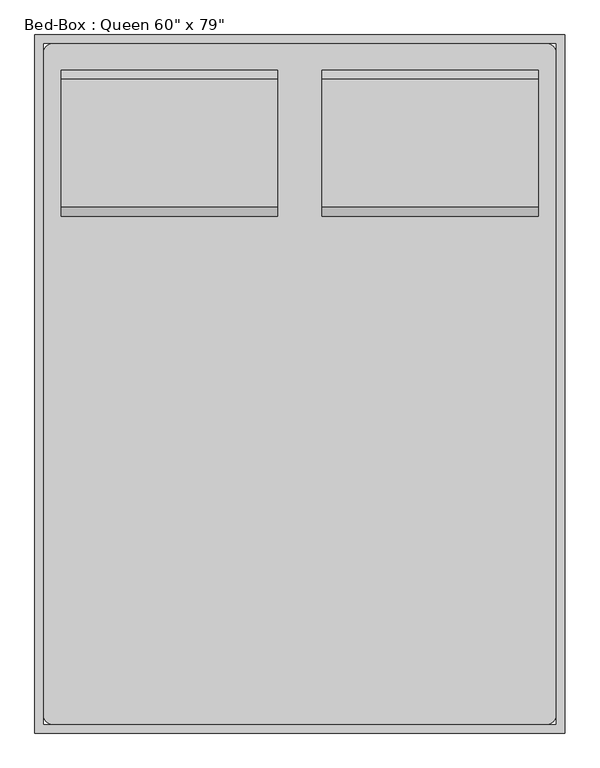
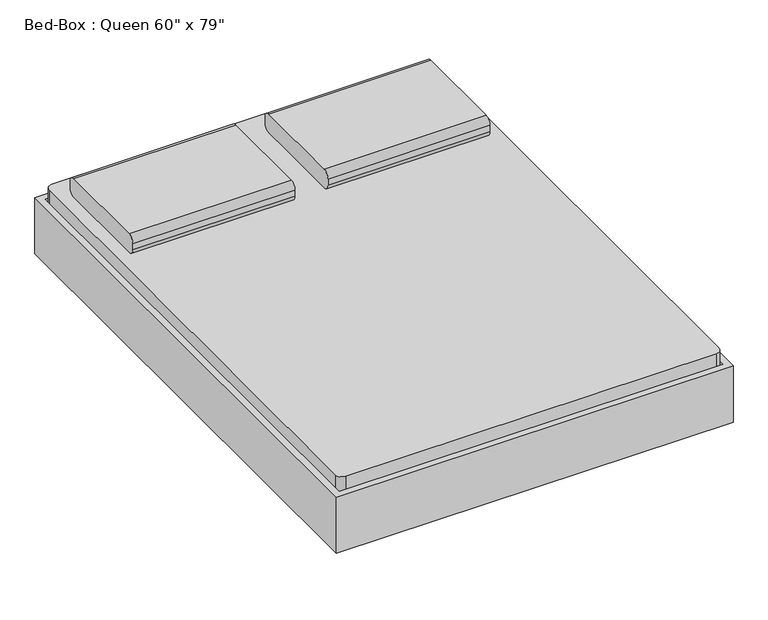
"""IFC4 building model written with IfcOpenShell, lengths in millimetres: furniture geometry."""

from ifc_helpers import new_model, si_unit, point, frame, frame_2d, origin, place, context, project, spatial, polyline, circle_curve, trimmed, segment, composite_curve, outline, extrude, source, transform, mapped, element, save
from ifc_brep_helpers import plane_surface, cylinder_surface, revolved_surface, advanced_brep


def furniture_1d2926bd(model_context):
    return source(origin(), model_context, "Body", "SolidModel", [
        extrude(outline(composite_curve([segment(polyline([(641.8704918, 406.4), (273.5704918, 406.4)]), True, "CONTINUOUS"), segment(trimmed(circle_curve(frame_2d((273.5704918, 431.8)), 25.4), [point((273.5704918, 406.4))], [point((248.1704918, 431.8))], False, "CARTESIAN"), True, "CONTINUOUS"), segment(polyline([(248.1704918, 431.8), (248.1704918, 457.2)]), True, "CONTINUOUS"), segment(trimmed(circle_curve(frame_2d((273.5704918, 457.2)), 25.4), [point((248.1704918, 457.2))], [point((273.5704918, 482.6))], False, "CARTESIAN"), True, "CONTINUOUS"), segment(polyline([(273.5704918, 482.6), (641.8704918, 482.6)]), True, "CONTINUOUS"), segment(trimmed(circle_curve(frame_2d((641.8704918, 457.2)), 25.4), [point((641.8704918, 482.6))], [point((667.2704918, 457.2))], False, "CARTESIAN"), True, "CONTINUOUS"), segment(polyline([(667.2704918, 457.2), (667.2704918, 431.8)]), True, "CONTINUOUS"), segment(trimmed(circle_curve(frame_2d((641.8704918, 431.8)), 25.4), [point((667.2704918, 431.8))], [point((641.8704918, 406.4))], False, "CARTESIAN"), True, "CONTINUOUS")], self_intersect=False)), frame((402.652459, 0.0, 0.0), z_axis=(1.0, 0.0, 0.0), x_axis=(0.0, 1.0, 0.0)), (0.0, 0.0, 1.0), 622.3),
        extrude(outline(composite_curve([segment(polyline([(641.8704918, 406.4), (273.5704918, 406.4)]), True, "CONTINUOUS"), segment(trimmed(circle_curve(frame_2d((273.5704918, 431.8)), 25.4), [point((273.5704918, 406.4))], [point((248.1704918, 431.8))], False, "CARTESIAN"), True, "CONTINUOUS"), segment(polyline([(248.1704918, 431.8), (248.1704918, 457.2)]), True, "CONTINUOUS"), segment(trimmed(circle_curve(frame_2d((273.5704918, 457.2)), 25.4), [point((248.1704918, 457.2))], [point((273.5704918, 482.6))], False, "CARTESIAN"), True, "CONTINUOUS"), segment(polyline([(273.5704918, 482.6), (641.8704918, 482.6)]), True, "CONTINUOUS"), segment(trimmed(circle_curve(frame_2d((641.8704918, 457.2)), 25.4), [point((641.8704918, 482.6))], [point((667.2704918, 457.2))], False, "CARTESIAN"), True, "CONTINUOUS"), segment(polyline([(667.2704918, 457.2), (667.2704918, 431.8)]), True, "CONTINUOUS"), segment(trimmed(circle_curve(frame_2d((641.8704918, 431.8)), 25.4), [point((667.2704918, 431.8))], [point((641.8704918, 406.4))], False, "CARTESIAN"), True, "CONTINUOUS")], self_intersect=False)), frame((-346.647541, 0.0, 0.0), z_axis=(1.0, 0.0, 0.0), x_axis=(0.0, 1.0, 0.0)), (0.0, 0.0, 1.0), 622.3),
        advanced_brep(
        [(-397.1231784, 514.8704918, 177.8), (-397.1231784, 438.6704918, 177.8), (-397.1231784, 438.6704918, 196.85), (-397.1231784, 514.8704918, 196.85), (-346.3231784, 514.8704918, 177.8), (-346.3231784, 438.6704918, 177.8), (-334.1869899, 438.6704918, 196.85), (-334.1869899, 514.8704918, 196.85), (-270.2523099, 514.8704918, 14.6654962), (-270.2523099, 438.6704918, 14.6654962), (-252.9871466, 438.6704918, 22.716374), (-252.9871466, 514.8704918, 22.716374), (-247.2320921, 438.6704918, 0.0), (-247.2320921, 514.8704918, 0.0), (-247.2320921, 438.6704918, 19.05), (-247.2320921, 514.8704918, 19.05), (-168.6195862, 514.8704918, 0.0), (-168.6195862, 438.6704918, 0.0), (-168.6195862, 438.6704918, 19.05), (-168.6195862, 514.8704918, 19.05), (-155.9195862, 438.6704918, 3.4029547), (-155.9195862, 514.8704918, 3.4029547), (-165.4445862, 438.6704918, 19.9007387), (-165.4445862, 514.8704918, 19.9007387), (-95.822541, 514.8704918, 38.1), (-95.822541, 438.6704918, 38.1), (-100.9269731, 438.6704918, 57.15), (-100.9269731, 514.8704918, 57.15), (774.4518216, 514.8704918, 38.1), (774.4518216, 438.6704918, 38.1), (779.5562537, 438.6704918, 57.15), (779.5562537, 514.8704918, 57.15), (834.5488669, 514.8704918, 3.4029547), (834.5488669, 438.6704918, 3.4029547), (844.0738669, 438.6704918, 19.9007387), (844.0738669, 514.8704918, 19.9007387), (847.2488669, 438.6704918, 0.0), (847.2488669, 514.8704918, 0.0), (847.2488669, 438.6704918, 19.05), (847.2488669, 514.8704918, 19.05), (925.8613728, 514.8704918, 0.0), (925.8613728, 438.6704918, 0.0), (925.8613728, 438.6704918, 19.05), (925.8613728, 514.8704918, 19.05), (948.8815906, 438.6704918, 14.6654962), (948.8815906, 514.8704918, 14.6654962), (931.6164272, 438.6704918, 22.716374), (931.6164272, 514.8704918, 22.716374), (1024.952459, 514.8704918, 177.8), (1024.952459, 438.6704918, 177.8), (1012.8162705, 438.6704918, 196.85), (1012.8162705, 514.8704918, 196.85), (1075.752459, 514.8704918, 177.8), (1075.752459, 514.8704918, 196.85), (1075.752459, 438.6704918, 196.85), (1075.752459, 438.6704918, 177.8)],
        [
            (0, 1),
            (1, 2),
            (2, 3),
            (3, 0),
            (0, 4),
            (4, 5),
            (5, 1),
            (5, 6),
            (6, 2),
            (6, 7),
            (7, 3),
            (7, 4),
            (4, 8),
            (8, 9),
            (9, 5),
            (9, 10),
            (10, 6),
            (10, 11),
            (11, 7),
            (11, 8),
            (12, 9, circle_curve(frame((-247.2320921, 438.6704918, 25.4), z_axis=(0.0, 1.0, 0.0), x_axis=(-0.9063077870366486, 0.0, -0.42261826174070233)), 25.4)),
            (8, 13, circle_curve(frame((-247.2320921, 514.8704918, 25.4), z_axis=(0.0, -1.0, 0.0), x_axis=(-0.9063077870366486, 0.0, -0.42261826174070233)), 25.4)),
            (13, 12),
            (14, 10, circle_curve(frame((-247.2320921, 438.6704918, 25.4), z_axis=(0.0, 1.0, 0.0), x_axis=(-0.9063077870366486, 0.0, -0.42261826174070233)), 6.35)),
            (12, 14),
            (15, 11, circle_curve(frame((-247.2320921, 514.8704918, 25.4), z_axis=(0.0, 1.0, 0.0), x_axis=(-0.9063077870366486, 0.0, -0.42261826174070233)), 6.35)),
            (14, 15),
            (15, 13),
            (13, 16),
            (16, 17),
            (17, 12),
            (17, 18),
            (18, 14),
            (18, 19),
            (19, 15),
            (19, 16),
            (20, 17, circle_curve(frame((-168.6195862, 438.6704918, 25.4), z_axis=(0.0, 1.0, 0.0), x_axis=(0.0, 0.0, -1.0)), 25.4)),
            (16, 21, circle_curve(frame((-168.6195862, 514.8704918, 25.4), z_axis=(0.0, -1.0, 0.0), x_axis=(0.0, 0.0, -1.0)), 25.4)),
            (21, 20),
            (22, 18, circle_curve(frame((-168.6195862, 438.6704918, 25.4), z_axis=(0.0, 1.0, 0.0), x_axis=(0.0, 0.0, -1.0)), 6.35)),
            (20, 22),
            (23, 19, circle_curve(frame((-168.6195862, 514.8704918, 25.4), z_axis=(0.0, 1.0, 0.0), x_axis=(0.0, 0.0, -1.0)), 6.35)),
            (22, 23),
            (23, 21),
            (21, 24),
            (24, 25),
            (25, 20),
            (25, 26),
            (26, 22),
            (26, 27),
            (27, 23),
            (27, 24),
            (24, 28),
            (28, 29),
            (29, 25),
            (29, 30),
            (30, 26),
            (30, 31),
            (31, 27),
            (31, 28),
            (28, 32),
            (32, 33),
            (33, 29),
            (33, 34),
            (34, 30),
            (34, 35),
            (35, 31),
            (35, 32),
            (36, 33, circle_curve(frame((847.2488669, 438.6704918, 25.4), z_axis=(0.0, 1.0, 0.0), x_axis=(-0.5000000000000463, 0.0, -0.8660254037844118)), 25.4)),
            (32, 37, circle_curve(frame((847.2488669, 514.8704918, 25.4), z_axis=(0.0, -1.0, 0.0), x_axis=(-0.5000000000000463, 0.0, -0.8660254037844118)), 25.4)),
            (37, 36),
            (38, 34, circle_curve(frame((847.2488669, 438.6704918, 25.4), z_axis=(0.0, 1.0, 0.0), x_axis=(-0.5000000000000463, 0.0, -0.8660254037844118)), 6.35)),
            (36, 38),
            (39, 35, circle_curve(frame((847.2488669, 514.8704918, 25.4), z_axis=(0.0, 1.0, 0.0), x_axis=(-0.5000000000000463, 0.0, -0.8660254037844118)), 6.35)),
            (38, 39),
            (39, 37),
            (37, 40),
            (40, 41),
            (41, 36),
            (41, 42),
            (42, 38),
            (42, 43),
            (43, 39),
            (43, 40),
            (44, 41, circle_curve(frame((925.8613728, 438.6704918, 25.4), z_axis=(0.0, 1.0, 0.0), x_axis=(0.0, 0.0, -1.0)), 25.4)),
            (40, 45, circle_curve(frame((925.8613728, 514.8704918, 25.4), z_axis=(0.0, -1.0, 0.0), x_axis=(0.0, 0.0, -1.0)), 25.4)),
            (45, 44),
            (46, 42, circle_curve(frame((925.8613728, 438.6704918, 25.4), z_axis=(0.0, 1.0, 0.0), x_axis=(0.0, 0.0, -1.0)), 6.35)),
            (44, 46),
            (47, 43, circle_curve(frame((925.8613728, 514.8704918, 25.4), z_axis=(0.0, 1.0, 0.0), x_axis=(0.0, 0.0, -1.0)), 6.35)),
            (46, 47),
            (47, 45),
            (45, 48),
            (48, 49),
            (49, 44),
            (49, 50),
            (50, 46),
            (50, 51),
            (51, 47),
            (51, 48),
            (52, 53),
            (53, 54),
            (54, 55),
            (55, 52),
            (48, 52),
            (55, 49),
            (54, 50),
            (53, 51),
        ],
        [
            plane_surface(frame((-397.1231784, 768.8704918, -152.9490627), z_axis=(-1.0, 0.0, 0.0), x_axis=(0.0, 1.0, 0.0))),
            plane_surface(frame((-397.1231784, 514.8704918, 177.8), z_axis=(0.0, 0.0, -1.0), x_axis=(1.0, 0.0, 0.0))),
            plane_surface(frame((-397.1231784, 438.6704918, 177.8), z_axis=(0.0, -1.0, 0.0), x_axis=(1.0, 0.0, 0.0))),
            plane_surface(frame((-397.1231784, 438.6704918, 196.85), z_axis=(0.0, 0.0, 1.0), x_axis=(1.0, 0.0, 0.0))),
            plane_surface(frame((-397.1231784, 514.8704918, 196.85), z_axis=(0.0, 1.0, 0.0), x_axis=(1.0, 0.0, 0.0))),
            plane_surface(frame((-346.3231784, 514.8704918, 177.8), z_axis=(-0.9063077870366485, 0.0, -0.4226182617407027), x_axis=(0.4226182617407027, 0.0, -0.9063077870366485))),
            plane_surface(frame((-346.3231784, 438.6704918, 177.8), z_axis=(0.0, -1.0, 0.0), x_axis=(0.4226182617407025, 0.0, -0.9063077870366486))),
            plane_surface(frame((-334.1869899, 438.6704918, 196.85), z_axis=(0.9063077870366484, 0.0, 0.4226182617407028), x_axis=(0.4226182617407028, 0.0, -0.9063077870366484))),
            plane_surface(frame((-334.1869899, 514.8704918, 196.85), z_axis=(0.0, 1.0, 0.0), x_axis=(0.42261826174070277, 0.0, -0.9063077870366485))),
            cylinder_surface(frame((-247.2320921, 768.8704918, 25.4), z_axis=(0.0, -1.0, 0.0), x_axis=(-0.9063077870366486, 0.0, -0.42261826174070233)), 25.4),
            plane_surface(frame((-247.2320921, 438.6704918, 25.4), z_axis=(0.0, -1.0, 0.0), x_axis=(-0.9063077870366486, 0.0, -0.42261826174070233))),
            revolved_surface(polyline([(-252.9871465476827, 438.6704918, 22.71637403794654), (-252.9871465476827, 514.8704918, 22.71637403794654)]), (-247.2320921, 768.8704918, 25.4), (0.0, -1.0, 0.0)),
            plane_surface(frame((-247.2320921, 514.8704918, 25.4), z_axis=(0.0, 1.0, 0.0), x_axis=(-0.9063077870366486, 0.0, -0.42261826174070233))),
            plane_surface(frame((-247.2320921, 514.8704918, 0.0), z_axis=(0.0, 0.0, -1.0), x_axis=(1.0, 0.0, 0.0))),
            plane_surface(frame((-247.2320921, 438.6704918, 0.0), z_axis=(0.0, -1.0, 0.0), x_axis=(1.0, 0.0, 0.0))),
            plane_surface(frame((-247.2320921, 438.6704918, 19.05), z_axis=(0.0, 0.0, 1.0), x_axis=(1.0, 0.0, 0.0))),
            plane_surface(frame((-247.2320921, 514.8704918, 19.05), z_axis=(0.0, 1.0, 0.0), x_axis=(1.0, 0.0, 0.0))),
            cylinder_surface(frame((-168.6195862, 768.8704918, 25.4), z_axis=(0.0, -1.0, 0.0), x_axis=(0.0, 0.0, -1.0)), 25.4),
            plane_surface(frame((-168.6195862, 438.6704918, 25.4), z_axis=(0.0, -1.0, 0.0), x_axis=(0.0, 0.0, -1.0))),
            revolved_surface(polyline([(-168.6195862, 438.6704918, 19.049999999999997), (-168.6195862, 514.8704918, 19.049999999999997)]), (-168.6195862, 768.8704918, 25.4), (0.0, -1.0, 0.0)),
            plane_surface(frame((-168.6195862, 514.8704918, 25.4), z_axis=(0.0, 1.0, 0.0), x_axis=(0.0, 0.0, -1.0))),
            plane_surface(frame((-155.9195862, 514.8704918, 3.4029547), z_axis=(0.49999999999988004, 0.0, -0.866025403784508), x_axis=(0.866025403784508, 0.0, 0.49999999999988004))),
            plane_surface(frame((-155.9195862, 438.6704918, 3.4029547), z_axis=(0.0, -1.0, 0.0), x_axis=(0.8660254037845078, 0.0, 0.49999999999988026))),
            plane_surface(frame((-165.4445862, 438.6704918, 19.9007387), z_axis=(-0.4999999999998799, 0.0, 0.866025403784508), x_axis=(0.866025403784508, 0.0, 0.4999999999998799))),
            plane_surface(frame((-165.4445862, 514.8704918, 19.9007387), z_axis=(0.0, 1.0, 0.0), x_axis=(0.8660254037845075, 0.0, 0.49999999999988076))),
            plane_surface(frame((-95.822541, 514.8704918, 38.1), z_axis=(0.0, 0.0, -1.0), x_axis=(1.0, 0.0, 0.0))),
            plane_surface(frame((-95.822541, 438.6704918, 38.1), z_axis=(0.0, -1.0, 0.0), x_axis=(1.0, 0.0, 0.0))),
            plane_surface(frame((-100.9269731, 438.6704918, 57.15), z_axis=(0.0, 0.0, 1.0), x_axis=(1.0, 0.0, 0.0))),
            plane_surface(frame((-100.9269731, 514.8704918, 57.15), z_axis=(0.0, 1.0, 0.0), x_axis=(1.0, 0.0, 0.0))),
            plane_surface(frame((774.4518216, 514.8704918, 38.1), z_axis=(-0.5000000000000455, 0.0, -0.8660254037844125), x_axis=(0.8660254037844125, 0.0, -0.5000000000000455))),
            plane_surface(frame((774.4518216, 438.6704918, 38.1), z_axis=(0.0, -1.0, 0.0), x_axis=(0.866025403784412, 0.0, -0.5000000000000463))),
            plane_surface(frame((779.5562537, 438.6704918, 57.15), z_axis=(0.5000000000000466, 0.0, 0.8660254037844117), x_axis=(0.8660254037844117, 0.0, -0.5000000000000466))),
            plane_surface(frame((779.5562537, 514.8704918, 57.15), z_axis=(0.0, 1.0, 0.0), x_axis=(0.8660254037844115, 0.0, -0.5000000000000471))),
            cylinder_surface(frame((847.2488669, 768.8704918, 25.4), z_axis=(0.0, -1.0, 0.0), x_axis=(-0.5000000000000463, 0.0, -0.8660254037844118)), 25.4),
            plane_surface(frame((847.2488669, 438.6704918, 25.4), z_axis=(0.0, -1.0000000000000002, 0.0), x_axis=(-0.5000000000000464, 0.0, -0.866025403784412))),
            revolved_surface(polyline([(844.0738668999998, 438.6704918, 19.90073868596898), (844.0738668999998, 514.8704918, 19.90073868596898)]), (847.2488669, 768.8704918, 25.4), (0.0, -1.0, 0.0)),
            plane_surface(frame((847.2488669, 514.8704918, 25.4), z_axis=(0.0, 1.0000000000000002, 0.0), x_axis=(-0.5000000000000464, 0.0, -0.866025403784412))),
            plane_surface(frame((847.2488669, 514.8704918, 0.0), z_axis=(0.0, 0.0, -1.0), x_axis=(1.0, 0.0, 0.0))),
            plane_surface(frame((847.2488669, 438.6704918, 0.0), z_axis=(0.0, -1.0, 0.0), x_axis=(1.0, 0.0, 0.0))),
            plane_surface(frame((847.2488669, 438.6704918, 19.05), z_axis=(0.0, 0.0, 1.0), x_axis=(1.0, 0.0, 0.0))),
            plane_surface(frame((847.2488669, 514.8704918, 19.05), z_axis=(0.0, 1.0, 0.0), x_axis=(1.0, 0.0, 0.0))),
            cylinder_surface(frame((925.8613728, 768.8704918, 25.4), z_axis=(0.0, -1.0, 0.0), x_axis=(0.0, 0.0, -1.0)), 25.4),
            plane_surface(frame((925.8613728, 438.6704918, 25.4), z_axis=(0.0, -1.0, 0.0), x_axis=(0.0, 0.0, -1.0))),
            revolved_surface(polyline([(925.8613728, 438.6704918, 19.049999999999997), (925.8613728, 514.8704918, 19.049999999999997)]), (925.8613728, 768.8704918, 25.4), (0.0, -1.0, 0.0)),
            plane_surface(frame((925.8613728, 514.8704918, 25.4), z_axis=(0.0, 1.0, 0.0), x_axis=(0.0, 0.0, -1.0))),
            plane_surface(frame((948.8815906, 514.8704918, 14.6654962), z_axis=(0.90630778703668, 0.0, -0.42261826174063505), x_axis=(0.42261826174063505, 0.0, 0.90630778703668))),
            plane_surface(frame((948.8815906, 438.6704918, 14.6654962), z_axis=(0.0, -1.0, 0.0), x_axis=(0.42261826174063566, 0.0, 0.9063077870366797))),
            plane_surface(frame((931.6164272, 438.6704918, 22.716374), z_axis=(-0.9063077870366801, 0.0, 0.42261826174063477), x_axis=(0.42261826174063477, 0.0, 0.9063077870366801))),
            plane_surface(frame((931.6164272, 514.8704918, 22.716374), z_axis=(0.0, 1.0, 0.0), x_axis=(0.4226182617406345, 0.0, 0.9063077870366802))),
            plane_surface(frame((1075.752459, 768.8704918, -152.9490627), z_axis=(1.0, 0.0, 0.0), x_axis=(0.0, 1.0, 0.0))),
            plane_surface(frame((1024.952459, 514.8704918, 177.8), z_axis=(0.0, 0.0, -1.0), x_axis=(1.0, 0.0, 0.0))),
            plane_surface(frame((1024.952459, 438.6704918, 177.8), z_axis=(0.0, -1.0, 0.0), x_axis=(1.0, 0.0, 0.0))),
            plane_surface(frame((1012.8162705, 438.6704918, 196.85), z_axis=(0.0, 0.0, 1.0), x_axis=(1.0, 0.0, 0.0))),
            plane_surface(frame((1012.8162705, 514.8704918, 196.85), z_axis=(0.0, 1.0, 0.0), x_axis=(1.0, 0.0, 0.0))),
        ],
        [
            (0, [[1, 2, 3, 4]]),
            (1, [[-1, 5, 6, 7]]),
            (2, [[-2, -7, 8, 9]]),
            (3, [[-3, -9, 10, 11]]),
            (4, [[-4, -11, 12, -5]]),
            (5, [[-6, 13, 14, 15]]),
            (6, [[-8, -15, 16, 17]]),
            (7, [[-10, -17, 18, 19]]),
            (8, [[-12, -19, 20, -13]]),
            (9, [[21, -14, 22, 23]]),
            (10, [[24, -16, -21, 25]]),
            (11, [[26, -18, -24, 27]]),
            (12, [[-22, -20, -26, 28]]),
            (13, [[-23, 29, 30, 31]]),
            (14, [[-25, -31, 32, 33]]),
            (15, [[-27, -33, 34, 35]]),
            (16, [[-28, -35, 36, -29]]),
            (17, [[37, -30, 38, 39]]),
            (18, [[40, -32, -37, 41]]),
            (19, [[42, -34, -40, 43]]),
            (20, [[-38, -36, -42, 44]]),
            (21, [[-39, 45, 46, 47]]),
            (22, [[-41, -47, 48, 49]]),
            (23, [[-43, -49, 50, 51]]),
            (24, [[-44, -51, 52, -45]]),
            (25, [[-46, 53, 54, 55]]),
            (26, [[-48, -55, 56, 57]]),
            (27, [[-50, -57, 58, 59]]),
            (28, [[-52, -59, 60, -53]]),
            (29, [[-54, 61, 62, 63]]),
            (30, [[-56, -63, 64, 65]]),
            (31, [[-58, -65, 66, 67]]),
            (32, [[-60, -67, 68, -61]]),
            (33, [[69, -62, 70, 71]]),
            (34, [[72, -64, -69, 73]]),
            (35, [[74, -66, -72, 75]]),
            (36, [[-70, -68, -74, 76]]),
            (37, [[-71, 77, 78, 79]]),
            (38, [[-73, -79, 80, 81]]),
            (39, [[-75, -81, 82, 83]]),
            (40, [[-76, -83, 84, -77]]),
            (41, [[85, -78, 86, 87]]),
            (42, [[88, -80, -85, 89]]),
            (43, [[90, -82, -88, 91]]),
            (44, [[-86, -84, -90, 92]]),
            (45, [[-87, 93, 94, 95]]),
            (46, [[-89, -95, 96, 97]]),
            (47, [[-91, -97, 98, 99]]),
            (48, [[-92, -99, 100, -93]]),
            (49, [[101, 102, 103, 104]]),
            (50, [[-94, 105, -104, 106]]),
            (51, [[-96, -106, -103, 107]]),
            (52, [[-98, -107, -102, 108]]),
            (53, [[-100, -108, -101, -105]]),
        ],
    ),
        extrude(outline(composite_curve([segment(polyline([(-372.047541, 743.4704918), (1050.352459, 743.4704918)]), True, "CONTINUOUS"), segment(trimmed(circle_curve(frame_2d((1050.352459, 718.0704918)), 25.4), [point((1050.352459, 743.4704918))], [point((1075.752459, 718.0704918))], False, "CARTESIAN"), True, "CONTINUOUS"), segment(polyline([(1075.752459, 718.0704918), (1075.752459, -1186.9295082)]), True, "CONTINUOUS"), segment(trimmed(circle_curve(frame_2d((1050.352459, -1186.9295082)), 25.4), [point((1075.752459, -1186.9295082))], [point((1050.352459, -1212.3295082))], False, "CARTESIAN"), True, "CONTINUOUS"), segment(polyline([(1050.352459, -1212.3295082), (-372.047541, -1212.3295082)]), True, "CONTINUOUS"), segment(trimmed(circle_curve(frame_2d((-372.047541, -1186.9295082)), 25.4), [point((-372.047541, -1212.3295082))], [point((-397.447541, -1186.9295082))], False, "CARTESIAN"), True, "CONTINUOUS"), segment(polyline([(-397.447541, -1186.9295082), (-397.447541, 718.0704918)]), True, "CONTINUOUS"), segment(trimmed(circle_curve(frame_2d((-372.047541, 718.0704918)), 25.4), [point((-397.447541, 718.0704918))], [point((-372.047541, 743.4704918))], False, "CARTESIAN"), True, "CONTINUOUS")], self_intersect=False)), frame((0.0, 0.0, 203.2), z_axis=(0.0, 0.0, 1.0), x_axis=(1.0, 0.0, 0.0)), (0.0, 0.0, 1.0), 203.2),
        advanced_brep(
        [(-397.447541, -932.9295082, 196.85), (-397.447541, -932.9295082, 177.8), (-397.447541, -1009.1295082, 177.8), (-397.447541, -1009.1295082, 196.85), (-334.5113525, -932.9295082, 196.85), (-346.647541, -932.9295082, 177.8), (-346.647541, -1009.1295082, 177.8), (-334.5113525, -1009.1295082, 196.85), (-253.3115092, -932.9295082, 22.716374), (-270.5766725, -932.9295082, 14.6654962), (-270.5766725, -1009.1295082, 14.6654962), (-253.3115092, -1009.1295082, 22.716374), (-247.5564547, -932.9295082, 0.0), (-247.5564547, -932.9295082, 19.05), (-247.5564547, -1009.1295082, 0.0), (-247.5564547, -1009.1295082, 19.05), (-168.9439489, -932.9295082, 19.05), (-168.9439489, -932.9295082, 0.0), (-168.9439489, -1009.1295082, 0.0), (-168.9439489, -1009.1295082, 19.05), (-156.2439489, -932.9295082, 3.4029547), (-165.7689489, -932.9295082, 19.9007387), (-156.2439489, -1009.1295082, 3.4029547), (-165.7689489, -1009.1295082, 19.9007387), (-101.2513357, -932.9295082, 57.15), (-96.1469036, -932.9295082, 38.1), (-96.1469036, -1009.1295082, 38.1), (-101.2513357, -1009.1295082, 57.15), (779.5562537, -932.9295082, 57.15), (774.4518216, -932.9295082, 38.1), (774.4518216, -1009.1295082, 38.1), (779.5562537, -1009.1295082, 57.15), (844.0738669, -932.9295082, 19.9007387), (834.5488669, -932.9295082, 3.4029547), (834.5488669, -1009.1295082, 3.4029547), (844.0738669, -1009.1295082, 19.9007387), (847.2488669, -932.9295082, 0.0), (847.2488669, -932.9295082, 19.05), (847.2488669, -1009.1295082, 0.0), (847.2488669, -1009.1295082, 19.05), (925.8613728, -932.9295082, 19.05), (925.8613728, -932.9295082, 0.0), (925.8613728, -1009.1295082, 0.0), (925.8613728, -1009.1295082, 19.05), (948.8815906, -932.9295082, 14.6654962), (931.6164272, -932.9295082, 22.716374), (948.8815906, -1009.1295082, 14.6654962), (931.6164272, -1009.1295082, 22.716374), (1012.8162705, -932.9295082, 196.85), (1024.952459, -932.9295082, 177.8), (1024.952459, -1009.1295082, 177.8), (1012.8162705, -1009.1295082, 196.85), (1075.752459, -932.9295082, 196.85), (1075.752459, -1009.1295082, 196.85), (1075.752459, -1009.1295082, 177.8), (1075.752459, -932.9295082, 177.8)],
        [
            (0, 1),
            (1, 2),
            (2, 3),
            (3, 0),
            (0, 4),
            (4, 5),
            (5, 1),
            (5, 6),
            (6, 2),
            (6, 7),
            (7, 3),
            (7, 4),
            (4, 8),
            (8, 9),
            (9, 5),
            (9, 10),
            (10, 6),
            (10, 11),
            (11, 7),
            (11, 8),
            (12, 9, circle_curve(frame((-247.5564547, -932.9295082, 25.4), z_axis=(0.0, 1.0, 0.0), x_axis=(-0.906307787036663, 0.0, -0.4226182617406713)), 25.4)),
            (8, 13, circle_curve(frame((-247.5564547, -932.9295082, 25.4), z_axis=(0.0, -1.0, 0.0), x_axis=(-0.906307787036663, 0.0, -0.4226182617406713)), 6.35)),
            (13, 12),
            (14, 10, circle_curve(frame((-247.5564547, -1009.1295082, 25.4), z_axis=(0.0, 1.0, 0.0), x_axis=(-0.906307787036663, 0.0, -0.4226182617406713)), 25.4)),
            (12, 14),
            (15, 11, circle_curve(frame((-247.5564547, -1009.1295082, 25.4), z_axis=(0.0, 1.0, 0.0), x_axis=(-0.906307787036663, 0.0, -0.4226182617406713)), 6.35)),
            (14, 15),
            (15, 13),
            (13, 16),
            (16, 17),
            (17, 12),
            (17, 18),
            (18, 14),
            (18, 19),
            (19, 15),
            (19, 16),
            (20, 17, circle_curve(frame((-168.9439489, -932.9295082, 25.4), z_axis=(0.0, 1.0, 0.0), x_axis=(0.0, 0.0, -1.0)), 25.4)),
            (16, 21, circle_curve(frame((-168.9439489, -932.9295082, 25.4), z_axis=(0.0, -1.0, 0.0), x_axis=(0.0, 0.0, -1.0)), 6.35)),
            (21, 20),
            (22, 18, circle_curve(frame((-168.9439489, -1009.1295082, 25.4), z_axis=(0.0, 1.0, 0.0), x_axis=(0.0, 0.0, -1.0)), 25.4)),
            (20, 22),
            (23, 19, circle_curve(frame((-168.9439489, -1009.1295082, 25.4), z_axis=(0.0, 1.0, 0.0), x_axis=(0.0, 0.0, -1.0)), 6.35)),
            (22, 23),
            (23, 21),
            (21, 24),
            (24, 25),
            (25, 20),
            (25, 26),
            (26, 22),
            (26, 27),
            (27, 23),
            (27, 24),
            (24, 28),
            (28, 29),
            (29, 25),
            (29, 30),
            (30, 26),
            (30, 31),
            (31, 27),
            (31, 28),
            (28, 32),
            (32, 33),
            (33, 29),
            (33, 34),
            (34, 30),
            (34, 35),
            (35, 31),
            (35, 32),
            (36, 33, circle_curve(frame((847.2488669, -932.9295082, 25.4), z_axis=(0.0, 1.0, 0.0), x_axis=(-0.5000000000000479, 0.0, -0.866025403784411)), 25.4)),
            (32, 37, circle_curve(frame((847.2488669, -932.9295082, 25.4), z_axis=(0.0, -1.0, 0.0), x_axis=(-0.5000000000000479, 0.0, -0.866025403784411)), 6.35)),
            (37, 36),
            (38, 34, circle_curve(frame((847.2488669, -1009.1295082, 25.4), z_axis=(0.0, 1.0, 0.0), x_axis=(-0.5000000000000479, 0.0, -0.866025403784411)), 25.4)),
            (36, 38),
            (39, 35, circle_curve(frame((847.2488669, -1009.1295082, 25.4), z_axis=(0.0, 1.0, 0.0), x_axis=(-0.5000000000000479, 0.0, -0.866025403784411)), 6.35)),
            (38, 39),
            (39, 37),
            (37, 40),
            (40, 41),
            (41, 36),
            (41, 42),
            (42, 38),
            (42, 43),
            (43, 39),
            (43, 40),
            (44, 41, circle_curve(frame((925.8613728, -932.9295082, 25.4), z_axis=(0.0, 1.0, 0.0), x_axis=(0.0, 0.0, -1.0)), 25.4)),
            (40, 45, circle_curve(frame((925.8613728, -932.9295082, 25.4), z_axis=(0.0, -1.0, 0.0), x_axis=(0.0, 0.0, -1.0)), 6.35)),
            (45, 44),
            (46, 42, circle_curve(frame((925.8613728, -1009.1295082, 25.4), z_axis=(0.0, 1.0, 0.0), x_axis=(0.0, 0.0, -1.0)), 25.4)),
            (44, 46),
            (47, 43, circle_curve(frame((925.8613728, -1009.1295082, 25.4), z_axis=(0.0, 1.0, 0.0), x_axis=(0.0, 0.0, -1.0)), 6.35)),
            (46, 47),
            (47, 45),
            (45, 48),
            (48, 49),
            (49, 44),
            (49, 50),
            (50, 46),
            (50, 51),
            (51, 47),
            (51, 48),
            (52, 53),
            (53, 54),
            (54, 55),
            (55, 52),
            (48, 52),
            (55, 49),
            (54, 50),
            (53, 51),
        ],
        [
            plane_surface(frame((-397.447541, -1237.7295082, -127.5947323), z_axis=(-1.0, 0.0, 0.0), x_axis=(0.0, 1.0, 0.0))),
            plane_surface(frame((-397.447541, -932.9295082, 196.85), z_axis=(0.0, 1.0, 0.0), x_axis=(1.0, 0.0, 0.0))),
            plane_surface(frame((-397.447541, -932.9295082, 177.8), z_axis=(0.0, 0.0, -1.0), x_axis=(1.0, 0.0, 0.0))),
            plane_surface(frame((-397.447541, -1009.1295082, 177.8), z_axis=(0.0, -1.0, 0.0), x_axis=(1.0, 0.0, 0.0))),
            plane_surface(frame((-397.447541, -1009.1295082, 196.85), z_axis=(0.0, 0.0, 1.0), x_axis=(1.0, 0.0, 0.0))),
            plane_surface(frame((-334.5113525, -932.9295082, 196.85), z_axis=(0.0, 1.0, 0.0), x_axis=(0.4226182617406707, 0.0, -0.9063077870366634))),
            plane_surface(frame((-346.647541, -932.9295082, 177.8), z_axis=(-0.9063077870366635, 0.0, -0.4226182617406707), x_axis=(0.4226182617406707, 0.0, -0.9063077870366635))),
            plane_surface(frame((-346.647541, -1009.1295082, 177.8), z_axis=(0.0, -1.0, 0.0), x_axis=(0.422618261740671, 0.0, -0.9063077870366633))),
            plane_surface(frame((-334.5113525, -1009.1295082, 196.85), z_axis=(0.9063077870366633, 0.0, 0.42261826174067113), x_axis=(0.42261826174067113, 0.0, -0.9063077870366633))),
            plane_surface(frame((-247.5564547, -932.9295082, 25.4), z_axis=(0.0, 1.0, 0.0), x_axis=(-0.906307787036663, 0.0, -0.4226182617406713))),
            cylinder_surface(frame((-247.5564547, -1237.7295082, 25.4), z_axis=(0.0, -1.0, 0.0), x_axis=(-0.906307787036663, 0.0, -0.4226182617406713)), 25.4),
            plane_surface(frame((-247.5564547, -1009.1295082, 25.4), z_axis=(0.0, -1.0, 0.0), x_axis=(-0.906307787036663, 0.0, -0.4226182617406713))),
            revolved_surface(polyline([(-253.3115091476828, -1009.1295082, 22.716374037946736), (-253.3115091476828, -932.9295082, 22.716374037946736)]), (-247.5564547, -1237.7295082, 25.4), (0.0, -1.0, 0.0)),
            plane_surface(frame((-247.5564547, -932.9295082, 19.05), z_axis=(0.0, 1.0, 0.0), x_axis=(1.0, 0.0, 0.0))),
            plane_surface(frame((-247.5564547, -932.9295082, 0.0), z_axis=(0.0, 0.0, -1.0), x_axis=(1.0, 0.0, 0.0))),
            plane_surface(frame((-247.5564547, -1009.1295082, 0.0), z_axis=(0.0, -1.0, 0.0), x_axis=(1.0, 0.0, 0.0))),
            plane_surface(frame((-247.5564547, -1009.1295082, 19.05), z_axis=(0.0, 0.0, 1.0), x_axis=(1.0, 0.0, 0.0))),
            plane_surface(frame((-168.9439489, -932.9295082, 25.4), z_axis=(0.0, 1.0, 0.0), x_axis=(0.0, 0.0, -1.0))),
            cylinder_surface(frame((-168.9439489, -1237.7295082, 25.4), z_axis=(0.0, -1.0, 0.0), x_axis=(0.0, 0.0, -1.0)), 25.4),
            plane_surface(frame((-168.9439489, -1009.1295082, 25.4), z_axis=(0.0, -1.0, 0.0), x_axis=(0.0, 0.0, -1.0))),
            revolved_surface(polyline([(-168.9439489, -1009.1295082, 19.049999999999997), (-168.9439489, -932.9295082, 19.049999999999997)]), (-168.9439489, -1237.7295082, 25.4), (0.0, -1.0, 0.0)),
            plane_surface(frame((-165.7689489, -932.9295082, 19.9007387), z_axis=(0.0, 1.0, 0.0), x_axis=(0.8660254037844788, 0.0, 0.4999999999999306))),
            plane_surface(frame((-156.2439489, -932.9295082, 3.4029547), z_axis=(0.49999999999993017, 0.0, -0.866025403784479), x_axis=(0.866025403784479, 0.0, 0.49999999999993017))),
            plane_surface(frame((-156.2439489, -1009.1295082, 3.4029547), z_axis=(0.0, -1.0, 0.0), x_axis=(0.8660254037844785, 0.0, 0.49999999999993106))),
            plane_surface(frame((-165.7689489, -1009.1295082, 19.9007387), z_axis=(-0.4999999999999309, 0.0, 0.8660254037844786), x_axis=(0.8660254037844786, 0.0, 0.4999999999999309))),
            plane_surface(frame((-101.2513357, -932.9295082, 57.15), z_axis=(0.0, 1.0, 0.0), x_axis=(1.0, 0.0, 0.0))),
            plane_surface(frame((-96.1469036, -932.9295082, 38.1), z_axis=(0.0, 0.0, -1.0), x_axis=(1.0, 0.0, 0.0))),
            plane_surface(frame((-96.1469036, -1009.1295082, 38.1), z_axis=(0.0, -1.0, 0.0), x_axis=(1.0, 0.0, 0.0))),
            plane_surface(frame((-101.2513357, -1009.1295082, 57.15), z_axis=(0.0, 0.0, 1.0), x_axis=(1.0, 0.0, 0.0))),
            plane_surface(frame((779.5562537, -932.9295082, 57.15), z_axis=(0.0, 1.0000000000000002, 0.0), x_axis=(0.8660254037844106, 0.0, -0.5000000000000487))),
            plane_surface(frame((774.4518216, -932.9295082, 38.1), z_axis=(-0.5000000000000477, 0.0, -0.8660254037844112), x_axis=(0.8660254037844112, 0.0, -0.5000000000000477))),
            plane_surface(frame((774.4518216, -1009.1295082, 38.1), z_axis=(0.0, -1.0000000000000002, 0.0), x_axis=(0.8660254037844105, 0.0, -0.500000000000049))),
            plane_surface(frame((779.5562537, -1009.1295082, 57.15), z_axis=(0.5000000000000498, 0.0, 0.8660254037844098), x_axis=(0.8660254037844098, 0.0, -0.5000000000000498))),
            plane_surface(frame((847.2488669, -932.9295082, 25.4), z_axis=(0.0, 1.0000000000000002, 0.0), x_axis=(-0.500000000000048, 0.0, -0.8660254037844111))),
            cylinder_surface(frame((847.2488669, -1237.7295082, 25.4), z_axis=(0.0, -1.0, 0.0), x_axis=(-0.5000000000000479, 0.0, -0.866025403784411)), 25.4),
            plane_surface(frame((847.2488669, -1009.1295082, 25.4), z_axis=(0.0, -1.0000000000000002, 0.0), x_axis=(-0.500000000000048, 0.0, -0.8660254037844111))),
            revolved_surface(polyline([(844.0738668999998, -1009.1295082, 19.90073868596899), (844.0738668999998, -932.9295082, 19.90073868596899)]), (847.2488669, -1237.7295082, 25.4), (0.0, -1.0, 0.0)),
            plane_surface(frame((847.2488669, -932.9295082, 19.05), z_axis=(0.0, 1.0, 0.0), x_axis=(1.0, 0.0, 0.0))),
            plane_surface(frame((847.2488669, -932.9295082, 0.0), z_axis=(0.0, 0.0, -1.0), x_axis=(1.0, 0.0, 0.0))),
            plane_surface(frame((847.2488669, -1009.1295082, 0.0), z_axis=(0.0, -1.0, 0.0), x_axis=(1.0, 0.0, 0.0))),
            plane_surface(frame((847.2488669, -1009.1295082, 19.05), z_axis=(0.0, 0.0, 1.0), x_axis=(1.0, 0.0, 0.0))),
            plane_surface(frame((925.8613728, -932.9295082, 25.4), z_axis=(0.0, 1.0, 0.0), x_axis=(0.0, 0.0, -1.0))),
            cylinder_surface(frame((925.8613728, -1237.7295082, 25.4), z_axis=(0.0, -1.0, 0.0), x_axis=(0.0, 0.0, -1.0)), 25.4),
            plane_surface(frame((925.8613728, -1009.1295082, 25.4), z_axis=(0.0, -1.0, 0.0), x_axis=(0.0, 0.0, -1.0))),
            revolved_surface(polyline([(925.8613728, -1009.1295082, 19.049999999999997), (925.8613728, -932.9295082, 19.049999999999997)]), (925.8613728, -1237.7295082, 25.4), (0.0, -1.0, 0.0)),
            plane_surface(frame((931.6164272, -932.9295082, 22.716374), z_axis=(0.0, 1.0, 0.0), x_axis=(0.4226182617405411, 0.0, 0.9063077870367238))),
            plane_surface(frame((948.8815906, -932.9295082, 14.6654962), z_axis=(0.9063077870367237, 0.0, -0.4226182617405414), x_axis=(0.4226182617405414, 0.0, 0.9063077870367237))),
            plane_surface(frame((948.8815906, -1009.1295082, 14.6654962), z_axis=(0.0, -1.0, 0.0), x_axis=(0.42261826174054123, 0.0, 0.9063077870367238))),
            plane_surface(frame((931.6164272, -1009.1295082, 22.716374), z_axis=(-0.9063077870367237, 0.0, 0.4226182617405414), x_axis=(0.4226182617405414, 0.0, 0.9063077870367237))),
            plane_surface(frame((1075.752459, -1237.7295082, -127.5947323), z_axis=(1.0, 0.0, 0.0), x_axis=(0.0, 1.0, 0.0))),
            plane_surface(frame((1012.8162705, -932.9295082, 196.85), z_axis=(0.0, 1.0, 0.0), x_axis=(1.0, 0.0, 0.0))),
            plane_surface(frame((1024.952459, -932.9295082, 177.8), z_axis=(0.0, 0.0, -1.0), x_axis=(1.0, 0.0, 0.0))),
            plane_surface(frame((1024.952459, -1009.1295082, 177.8), z_axis=(0.0, -1.0, 0.0), x_axis=(1.0, 0.0, 0.0))),
            plane_surface(frame((1012.8162705, -1009.1295082, 196.85), z_axis=(0.0, 0.0, 1.0), x_axis=(1.0, 0.0, 0.0))),
        ],
        [
            (0, [[1, 2, 3, 4]]),
            (1, [[-1, 5, 6, 7]]),
            (2, [[-2, -7, 8, 9]]),
            (3, [[-3, -9, 10, 11]]),
            (4, [[-4, -11, 12, -5]]),
            (5, [[-6, 13, 14, 15]]),
            (6, [[-8, -15, 16, 17]]),
            (7, [[-10, -17, 18, 19]]),
            (8, [[-12, -19, 20, -13]]),
            (9, [[21, -14, 22, 23]]),
            (10, [[24, -16, -21, 25]]),
            (11, [[26, -18, -24, 27]]),
            (12, [[-22, -20, -26, 28]]),
            (13, [[-23, 29, 30, 31]]),
            (14, [[-25, -31, 32, 33]]),
            (15, [[-27, -33, 34, 35]]),
            (16, [[-28, -35, 36, -29]]),
            (17, [[37, -30, 38, 39]]),
            (18, [[40, -32, -37, 41]]),
            (19, [[42, -34, -40, 43]]),
            (20, [[-38, -36, -42, 44]]),
            (21, [[-39, 45, 46, 47]]),
            (22, [[-41, -47, 48, 49]]),
            (23, [[-43, -49, 50, 51]]),
            (24, [[-44, -51, 52, -45]]),
            (25, [[-46, 53, 54, 55]]),
            (26, [[-48, -55, 56, 57]]),
            (27, [[-50, -57, 58, 59]]),
            (28, [[-52, -59, 60, -53]]),
            (29, [[-54, 61, 62, 63]]),
            (30, [[-56, -63, 64, 65]]),
            (31, [[-58, -65, 66, 67]]),
            (32, [[-60, -67, 68, -61]]),
            (33, [[69, -62, 70, 71]]),
            (34, [[72, -64, -69, 73]]),
            (35, [[74, -66, -72, 75]]),
            (36, [[-70, -68, -74, 76]]),
            (37, [[-71, 77, 78, 79]]),
            (38, [[-73, -79, 80, 81]]),
            (39, [[-75, -81, 82, 83]]),
            (40, [[-76, -83, 84, -77]]),
            (41, [[85, -78, 86, 87]]),
            (42, [[88, -80, -85, 89]]),
            (43, [[90, -82, -88, 91]]),
            (44, [[-86, -84, -90, 92]]),
            (45, [[-87, 93, 94, 95]]),
            (46, [[-89, -95, 96, 97]]),
            (47, [[-91, -97, 98, 99]]),
            (48, [[-92, -99, 100, -93]]),
            (49, [[101, 102, 103, 104]]),
            (50, [[-94, 105, -104, 106]]),
            (51, [[-96, -106, -103, 107]]),
            (52, [[-98, -107, -102, 108]]),
            (53, [[-100, -108, -101, -105]]),
        ],
    ),
        extrude(outline(polyline([(1101.152459, 768.8704918), (1101.152459, -1237.7295082), (-422.847541, -1237.7295082), (-422.847541, 768.8704918), (1101.152459, 768.8704918)]), holes=[polyline([(1075.752459, 743.4704918), (-397.447541, 743.4704918), (-397.447541, -1212.3295082), (1075.752459, -1212.3295082), (1075.752459, 743.4704918)])]), frame((0.0, 0.0, 127.0), z_axis=(0.0, 0.0, 1.0), x_axis=(1.0, 0.0, 0.0)), (0.0, 0.0, 1.0), 228.6),
    ])


if __name__ == "__main__":
    model = new_model("IFC4")
    model_context = context("Model", 3, world=origin())
    ifc_project = project(units=[si_unit("LENGTHUNIT", "METRE", prefix="MILLI")], contexts=[model_context])
    site = spatial("IfcSite", under=ifc_project)
    building = spatial("IfcBuilding", under=site)
    placement = place(None, origin())
    furniture_shape = furniture_1d2926bd(model_context)
    element("IfcFurniture", 1, ObjectType="Bed-Box : Queen 60\" x 79\"", at=placement, inside=building, context=model_context, shape_type="MappedRepresentation", body=[
        mapped(furniture_shape, transform((0.0, 0.0, 0.0), x_axis=(1.0, 0.0, 0.0), y_axis=(0.0, 1.0, 0.0), z_axis=(0.0, 0.0, 1.0))),
    ])
    save(model, "model.ifc")

# Revit data of these elements
# Type "Bed-Box : Queen 60\" x 79\""
#   Assembly Code = "E2020200"
#   Length = 6' - 7"
#   Width = 5' - 0"
#   Frame Material = Birch
#   Mattress Material = Linen, White
#   Default Elevation = 0
# Element 1 (IfcFurniture, "Bed-Box : Queen 60\" x 79\"")
#   Materials on its faces: "Birch", "Linen, White"
# Materials
#   "Birch": class "Wood", colour RGB 224 178 126, transparency 0, Description = "Betula Alleghaniensis", Cost = 0
#   "Linen, White": class "Textile", colour RGB 247 247 239, transparency 0, Description = "Linen, white", Cost = 0
